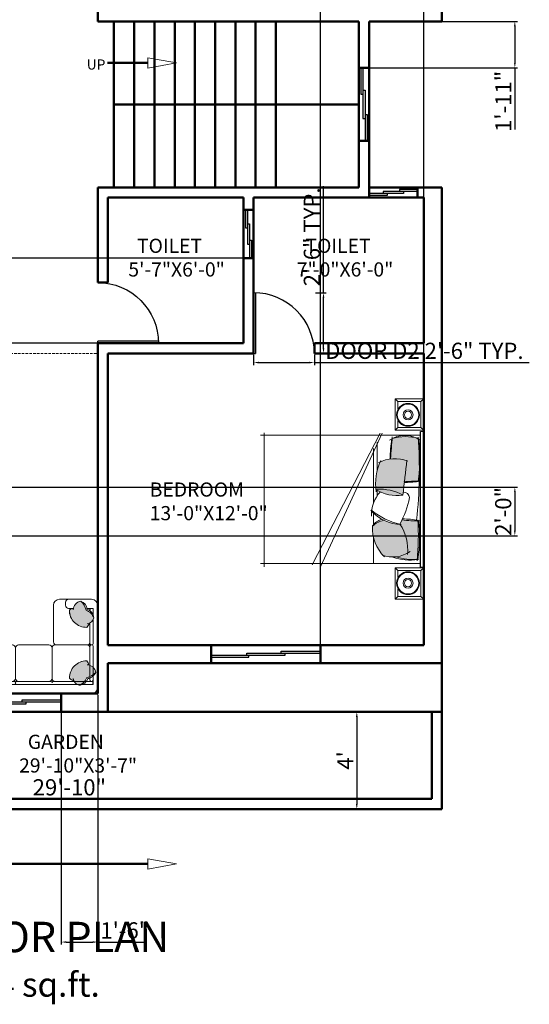
# Model space of a CAD drawing. Units: inches. Extents: x 1913 to 5309, y 1003 to 1733.
# Tile 7 of 23: x 2303 to 2555, y 1003 to 1489. Entities that reach past the tile are written whole.
import ezdxf

# ---------------------------------------------------------------- set-up
doc = ezdxf.new("R2010")
doc.units = ezdxf.units.IN
doc.linetypes.add('HIDDEN2', pattern=[0.1875, 0.125, -0.0625])
for name, color, linetype, lineweight in [('0.10', 252, 'Continuous', 9), ('0.15', 34, 'Continuous', 15), ('A-ANNO-DIMS', 2, 'Continuous', 18), ('A-ANNO-SYMB', 1, 'Continuous', 18), ('A-ANNO-TEXT', 7, 'Continuous', 18), ('A-AREA-IDEN', 3, 'Continuous', 18), ('A-DOOR', 4, 'Continuous', 25), ('A-FURN', 8, 'Continuous', 18), ('A-FURN-PATT', 8, 'Continuous', 13), ('A-GLAZ', 5, 'Continuous', 25), ('A-WALL', 7, 'Continuous', 50), ('A-WALL-OVHD', 8, 'HIDDEN2', 18)]:
    doc.layers.add(name, color=color, linetype=linetype, lineweight=lineweight)
doc.styles.get("Standard").update_dxf_attribs({"font": 'arial.ttf'})
doc.dimstyles.new('ISO-25', dxfattribs={"dimtxt": 8, "dimasz": 2.5, "dimexe": 1.25, "dimexo": 0.625, "dimtad": 1, "dimdec": 1, "dimlunit": 3, "dimtxsty": 'Standard', "dimcen": 2.5, "dimclrd": 256, "dimclrt": 1, "dimadec": 0, "dimazin": 0, "dimtfac": 1, "dimtdec": 1, "dimtmove": 0, "dimatfit": 3, "dimfxl": 1, "dimarcsym": 0})

# ---------------------------------------------------------------- blocks, each defined once
blk = doc.blocks.new("D2 2'6")
for p, q in [((0, 30), (0, 0)), ((1, 30), (1, 0)), ((0, 0), (1, 0))]:
    blk.add_line(p, q)
blk.add_arc((0, 0), 30, 0, 90)
blk = doc.blocks.new('camita')
at = {"layer": '0.10'}
for p, q in [((-0.85, -0.045), (0.85, -0.045)), ((-0.805, -0.045), (-0.805, -2.048)), ((0.805, -0.045), (0.805, -2.048)), ((-0.827, -0.521), (0.846, -1.293)), ((-0.827, -0.548), (0.824, -1.399)), ((-0.716, -0.585), (-0.355, -0.585)), ((-0.114, -0.585), (-0.049, -0.585)), ((-0.638, -0.63), (0.043, -0.63)), ((0.175, -0.63), (0.318, -0.63)), ((0.474, -0.63), (0.805, -0.63)), ((-0.835, -2), (0.846, -2))]:
    blk.add_line(p, q, dxfattribs=at)
blk.add_lwpolyline([(-0.85, -0.041), (0.85, -0.041), (0.85, 0), (-0.85, 0)], close=True, dxfattribs=at)
for centre, radius, start, end in [((-0.457, -0.236), 0.344, 147.51, 213.8336), ((-0.2, -0.227), 0.586, 163.9263, 197.1409), ((-0.364, -5.846), 5.791, 83.8073, 94.1211), ((-0.51, -1.723), 1.678, 80.1255, 98.6619), ((2.353, -0.053), 2.58, 180.1063, 184.3854), ((-1.544, -0.245), 1.333, 359.9394, 7.5533), ((1.581, -0.289), 1.335, 170.3802, 178.9914), ((-1.44, -0.061), 1.712, 352.9291, 0.3959), ((0.452, -3.067), 3, 83.9026, 93.6759), ((0.486, -1.629), 1.578, 80.1602, 98.06), ((0.029, -0.138), 0.726, 342.5841, 6.0048), ((0.133, -0.17), 0.631, 339.923, 8.7433), ((-0.054, -0.363), 0.454, 159.3026, 206.5026), ((-1.33, -9.675), 9.499, 82.2708, 84.9399), ((-0.007, -0.258), 0.0828, 100.018, 179.736), ((-0.293, -1.438), 1.29, 61.9749, 77.8435), ((0.627, -0.752), 0.551, 82.9691, 124.6739), ((0.32, -0.394), 0.404, 341.4524, 33.4512), ((0.458, -0.545), 0.584, 151.0456, 184.1497), ((-0.534, -0.339), 0.487, 327.2644, 9.0473), ((-0.199, -0.274), 0.516, 310.7395, 359.0576), ((-0.567, -0.087), 0.906, 321.6953, 346.4626), ((-1.867, -14.986), 14.632, 84.6597, 85.7516), ((-0.46, 1.486), 1.909, 260.953, 268.6517), ((0.361, -0.133), 0.51, 267.2589, 315.2997), ((-0.2, 0.064), 0.667, 244.7809, 279.0606), ((0.179, -0.272), 0.383, 224.5284, 275.2229), ((0.438, -0.483), 0.19, 193.6849, 236.7035), ((0.571, -0.432), 0.315, 192.9388, 221.9636)]:
    blk.add_arc(centre, radius, start, end, dxfattribs=at)
blk = doc.blocks.new('VELADOR')
at = {"layer": '0.15'}
for p, q in [((-0.248, 0), (-0.203, -0.045)), ((0.248, 0), (0.202, -0.045)), ((-0.203, -0.405), (-0.248, -0.45)), ((0.248, -0.45), (0.202, -0.405))]:
    blk.add_line(p, q, dxfattribs=at)
blk.add_lwpolyline([(-0.248, 0), (-0.248, -0.45), (0.248, -0.45), (0.248, 0)], close=True, dxfattribs=at)
blk.add_lwpolyline([(0.092, -0.405), (0.202, -0.405), (0.202, -0.045), (-0.203, -0.045), (-0.203, -0.405), (-0.082, -0.405)], dxfattribs=at)
for radius in [0.18, 0.169, 0.0788, 0.0563]:
    blk.add_circle((0.005, -0.247), radius, dxfattribs=at)
blk = doc.blocks.new('SOFA 1')
at = {"transparency": 33554687}
h = blk.add_hatch(color=256, dxfattribs=at)
h.dxf.hatch_style = 1
h.paths.add_polyline_path([(3723.52, 1308.63, 0.147724), (3717.76, 1305.24, 0.310469), (3722.42, 1300.4), (3722.42, 1300.25, 0.156703), (3723.62, 1297.8, 0.425821), (3734.69, 1309.08, 0.121928), (3732.05, 1310.63, 0.233216), (3728.6, 1313.59, 0.213835)])
h = blk.add_hatch(color=256, dxfattribs=at)
h.dxf.hatch_style = 1
h.paths.add_polyline_path([(3769.65, 1307.6, 0.084911), (3767.15, 1309.12, 0.046133), (3766.46, 1311.13), (3759.18, 1311.13, 0.039409), (3758.92, 1310.24, 0.165523), (3756.31, 1309.02, 0.42585), (3767.59, 1297.95, 0.121928), (3769.15, 1300.58, 0.027403), (3769.65, 1300.83)])
h.paths.add_polyline_path([(3765.34, 1313.08), (3760.4, 1313.08, 0.097704), (3759.18, 1311.13), (3766.46, 1311.13, 0.04873)])
h.paths.add_polyline_path([(3763.76, 1314.88, 0.16488), (3760.4, 1313.08), (3765.34, 1313.08, 0.051917)])
h.paths.add_polyline_path([(3771.6, 1305.17, 0.090388), (3769.65, 1307.6), (3769.65, 1300.83, 0.136035), (3771.6, 1302.77)])
h = blk.add_hatch(color=256, dxfattribs=at)
h.dxf.hatch_style = 1
h.paths.add_polyline_path([(3769.16, 1235.96, 0.122267), (3767.6, 1238.61, 0.425972), (3756.32, 1227.54, 0.165563), (3758.93, 1226.32, 0.309481), (3763.76, 1221.69, 0.002677), (3763.83, 1221.72, 0.146094), (3767.16, 1227.43, 0.212433), (3772.1, 1232.48, 0.235342)])
h = blk.add_hatch(color=256, dxfattribs=at)
h.dxf.hatch_style = 1
h.paths.add_polyline_path([(3769.16, 1225.36, 0.122267), (3767.6, 1228.01, 0.425972), (3756.32, 1216.94, 0.165563), (3758.93, 1215.72, 0.309481), (3763.76, 1211.09, 0.002677), (3763.83, 1211.12, 0.146094), (3767.16, 1216.83, 0.212433), (3772.1, 1221.88, 0.235342)])
for p, q in [((3720.45, 1316.13), (3773.58, 1316.13)), ((3777.51, 1312.19), (3777.51, 1213.72))]:
    blk.add_line(p, q, dxfattribs=at)
for points in [[(3716.51, 1312.2), (3716.51, 1291.44)], [(3722.42, 1313.08), (3722.42, 1309.23), (3722.42, 1313.08), (3726.57, 1313.08)], [(3723.21, 1311.13), (3723.93, 1311.13)], [(3729.85, 1313.08), (3745.25, 1313.08)], [(3731.82, 1311.13), (3745.25, 1311.13)], [(3746.01, 1312.3), (3746.01, 1288.55)], [(3746.01, 1310.97), (3746.01, 1311.36)], [(3768.11, 1313.08), (3746.78, 1313.08)], [(3768.87, 1311.13), (3746.78, 1311.13)], [(3771.6, 1313.08), (3767.75, 1313.08), (3771.6, 1313.08), (3771.6, 1308.93)], [(3769.66, 1287.39), (3769.65, 1312.3)], [(3771.6, 1313.08), (3771.61, 1233.74)], [(3746.01, 1288.54), (3746.01, 1308.23)], [(3769.65, 1309.43), (3769.65, 1308.71)], [(3722.42, 1300.39), (3722.42, 1297.33)], [(3720.45, 1295.38), (3718.48, 1295.38)], [(3720.45, 1287.5), (3744.09, 1287.5)], [(3747.99, 1286.6), (3767.69, 1286.6)], [(3769.66, 1263.75), (3769.66, 1285.81)], [(3746.02, 1284.63), (3746.02, 1264.94)], [(3769.66, 1277.18), (3769.66, 1263.75)], [(3746.02, 1260.99), (3746.02, 1241.3)], [(3747.99, 1262.97), (3767.69, 1262.97)], [(3769.66, 1240.12), (3769.66, 1262.18)], [(3770.43, 1262.97), (3770.82, 1262.97)], [(3746.02, 1237.36), (3746.02, 1213.74)], [(3747.99, 1239.33), (3767.69, 1239.33)], [(3769.66, 1235.71), (3769.66, 1238.54)], [(3770.43, 1239.33), (3770.82, 1239.33)], [(3769.66, 1225.11), (3769.66, 1227.82)], [(3771.61, 1223.14), (3771.61, 1230.47)], [(3755.86, 1215.72), (3758.92, 1215.72)], [(3767.76, 1215.72), (3771.61, 1215.72), (3771.61, 1219.84), (3771.61, 1215.72)], [(3769.66, 1216.5), (3769.66, 1217.22)], [(3749.97, 1209.8), (3773.58, 1209.8)], [(3753.91, 1211.77), (3753.91, 1213.74)]]:
    blk.add_lwpolyline(points, close=True, dxfattribs=at)
for points in [[(3717.76, 1305.24, -0.147724), (3723.52, 1308.63, -0.213355), (3728.59, 1313.59, 0.213355), (3723.52, 1308.63, 0.147724), (3717.76, 1305.24, -0.249545), (3722.86, 1309.34, 0.249545), (3717.75, 1305.25, 0.356779), (3723.4, 1300.28, -0.356779), (3717.76, 1305.24)], [(3734.69, 1309.08, -0.425972), (3723.62, 1297.8, -0.165552), (3722.4, 1300.4, 0.165552), (3723.62, 1297.79, 0.425972), (3734.69, 1309.07, 0.121514), (3732.07, 1310.63, -0.121514), (3734.69, 1309.08)], [(3728.58, 1313.6, -0.306333), (3732.42, 1309.31, 0.306333), (3728.58, 1313.6, 0.306674), (3722.72, 1308.89, -0.306674), (3728.58, 1313.6)], [(3763.76, 1314.88, -0.147724), (3767.15, 1309.12, -0.213355), (3772.1, 1304.05, 0.213355), (3767.15, 1309.12, 0.147724), (3763.76, 1314.88, -0.249545), (3767.86, 1309.77, 0.249545), (3763.77, 1314.89, 0.356779), (3758.8, 1309.23, -0.356779), (3763.76, 1314.88)], [(3767.6, 1297.95, -0.425972), (3756.31, 1309.01, -0.165552), (3758.92, 1310.24, 0.165552), (3756.31, 1309.02, 0.425972), (3767.59, 1297.95, 0.121514), (3769.14, 1300.57, -0.121514), (3767.6, 1297.95)], [(3772.11, 1304.06, -0.306333), (3767.83, 1300.22, 0.306333), (3772.11, 1304.06, 0.306674), (3767.4, 1309.91, -0.306674), (3772.11, 1304.06)], [(3770.44, 1286.63, -0.414214), (3769.66, 1287.4, 0.414214), (3770.44, 1286.63, 0.414214), (3769.66, 1285.83, -0.414214), (3770.44, 1286.63)], [(3748.01, 1262.99, -0.414214), (3746.05, 1264.95, 0.414214), (3748.01, 1262.97, 0.414213), (3746.05, 1261.01, -0.414213), (3748.01, 1262.99)], [(3770.44, 1262.99, -0.414214), (3769.66, 1263.77, 0.414214), (3770.44, 1262.99, 0.414214), (3769.66, 1262.19, -0.414214), (3770.44, 1262.99)], [(3770.83, 1262.97, -0.414214), (3771.61, 1262.19, 0.414214), (3770.83, 1262.99, 0.414214), (3771.61, 1263.77, -0.414214), (3770.83, 1262.97)], [(3748.01, 1239.35, -0.414214), (3746.05, 1241.31, 0.414214), (3748.01, 1239.33, 0.414213), (3746.05, 1237.37, -0.414213), (3748.01, 1239.35)], [(3767.7, 1239.33, -0.414214), (3769.66, 1237.37, 0.414214), (3767.7, 1239.35, 0.414214), (3769.66, 1241.31, -0.414214), (3767.7, 1239.33)], [(3756.32, 1227.54, -0.425972), (3767.6, 1238.61, -0.121514), (3769.16, 1235.98, 0.121514), (3767.6, 1238.61, 0.425972), (3756.32, 1227.54, 0.165552), (3758.93, 1226.32, -0.165552), (3756.32, 1227.54)], [(3772.1, 1232.5, -0.306674), (3767.41, 1226.64, 0.306674), (3772.1, 1232.5, 0.306333), (3767.84, 1236.34, -0.306333), (3772.1, 1232.5)], [(3770.44, 1239.35, -0.414214), (3769.66, 1240.13, 0.414214), (3770.44, 1239.33, 0.414214), (3769.66, 1238.55, -0.414214), (3770.44, 1239.35)], [(3770.83, 1239.33, -0.414214), (3771.61, 1238.55, 0.414214), (3770.83, 1239.35, 0.414214), (3771.61, 1240.13, -0.414214), (3770.83, 1239.33)], [(3763.78, 1221.67, 0.249545), (3767.87, 1226.78, -0.249545), (3763.76, 1221.69, -0.356779), (3758.81, 1227.32, 0.356779), (3763.77, 1221.68, 0.147724), (3767.16, 1227.43, 0.213355), (3772.11, 1232.51, -0.213355), (3767.16, 1227.43, -0.147724), (3763.78, 1221.67)], [(3756.32, 1216.94, -0.200233), (3759.49, 1224.76, 0.200233), (3756.32, 1216.94, 0.165552), (3758.93, 1215.72, -0.165552), (3756.32, 1216.94)], [(3772.1, 1221.9, -0.306674), (3767.41, 1216.04, 0.306674), (3772.1, 1221.9, -0.213355), (3767.16, 1216.83, -0.147724), (3763.77, 1211.08, 0.147724), (3767.15, 1216.83, 0.213355), (3772.1, 1221.9)], [(3763.76, 1211.09, -0.356779), (3758.81, 1216.72, 0.356779), (3763.76, 1211.09, 0.249545), (3767.87, 1216.18, -0.249545), (3763.76, 1211.09)]]:
    blk.add_lwpolyline(points, format="xyb", dxfattribs=at)
for points in [[(3722.42, 1311.91, 0.414214), (3723.2, 1311.13, -0.414214)], [(3770.43, 1313.08, 0.414214), (3769.65, 1312.3, -0.414214)], [(3771.6, 1312.3, 0.414214), (3770.82, 1313.08, -0.414214)], [(3716.51, 1297.34, 0.414214), (3718.47, 1295.38, -0.414214)], [(3716.51, 1291.45, 0.414212), (3720.44, 1287.52, -0.414212)], [(3720.44, 1295.38, 0.414214), (3722.4, 1297.34, -0.414214)], [(3746.03, 1288.56, 0.414214), (3747.99, 1286.6, 0.414213), (3746.03, 1284.64, -0.414213), (3747.99, 1286.6, -0.414214)], [(3769.66, 1284.64, 0.414214), (3767.7, 1286.6, 0.414214), (3769.66, 1288.56, -0.414214), (3767.7, 1286.6, -0.414214)], [(3769.66, 1261.01, 0.414214), (3767.7, 1262.97, 0.414214), (3769.66, 1264.93, -0.414214), (3767.7, 1262.97, -0.414214)], [(3772.13, 1221.9, 0.306333), (3767.84, 1225.74, -0.306333)], [(3769.16, 1225.36, 0.071861), (3768.39, 1227.01, -0.071861)], [(3755.87, 1215.72, 0.414214), (3753.91, 1213.76, -0.414214)], [(3769.66, 1216.52, 0.414214), (3770.44, 1215.74, -0.414214)], [(3770.83, 1215.74, 0.414214), (3771.61, 1216.52, -0.414214)], [(3746.05, 1213.76, 0.414212), (3749.98, 1209.82, -0.414212)], [(3755.87, 1209.8, -0.414214), (3753.91, 1211.76, 0.414214)]]:
    blk.add_lwpolyline(points, format="xyb", close=True, dxfattribs=at)
for centre, radius, start, end in [((3720.44, 1312.2), 3.93, 90.00019, 179.99981), ((3720.44, 1312.19), 3.94, 89.91581, 179.91542), ((3744.09, 1309.21), 1.92, 358.76597, 90.51112), ((3745.22, 1312.29), 0.789, 0.84252, 90.84253), ((3745.24, 1311.91), 0.777, 270, 0), ((3745.24, 1311.91), 0.777, 270, 0), ((3746.8, 1312.29), 0.789, 89.15747, 179.15748), ((3746.79, 1311.91), 0.777, 180, 270), ((3746.79, 1311.91), 0.777, 180, 270), ((3747.93, 1309.21), 1.92, 89.48888, 181.23403), ((3768.87, 1312.3), 0.777, 360, 90), ((3768.87, 1311.91), 0.777, 270, 0), ((3773.58, 1312.2), 3.93, 0.00019, 89.99981), ((3773.57, 1312.19), 3.94, 359.91581, 89.91542), ((3744.08, 1289.48), 1.96, 270, 360), ((3744.08, 1289.48), 1.96, 270, 360), ((3773.58, 1213.73), 3.93, 270.00019, 359.99981), ((3773.59, 1213.73), 3.93, 269.91556, 359.91517)]:
    blk.add_arc(centre, radius, start, end, dxfattribs=at)
blk = doc.blocks.new('*D25')
at = {"layer": 'A-ANNO-DIMS', "color": 0, "lineweight": -2, "transparency": 16777216}
for p, q in [((2469.32, 1144.46), (2469.32, 1101.46)), ((2469.94, 1146.96), (2470.57, 1146.96)), ((2469.94, 1098.96), (2470.57, 1098.96))]:
    blk.add_line(p, q, dxfattribs=at)
at = {"layer": 'A-ANNO-DIMS', "color": 0, "transparency": 16777216}
for points in [[(2468.9, 1144.46), (2469.73, 1144.46), (2469.32, 1146.96)], [(2468.9, 1101.46), (2469.73, 1101.46), (2469.32, 1098.96)]]:
    blk.add_solid(points, dxfattribs=at)
at = {"layer": 'Defpoints', "color": 0, "transparency": 16777216}
for p in [(2469.32, 1146.96), (2469.32, 1098.96), (2469.32, 1098.96)]:
    blk.add_point(p, dxfattribs=at)
at = {"layer": 'A-ANNO-DIMS', "color": 0, "transparency": 16777216, "insert": (2464.69, 1122.96), "char_height": 8, "attachment_point": 5, "rotation": 90}
blk.add_mtext("4'", dxfattribs=at)
blk = doc.blocks.new('*D21')
at = {"layer": 'A-ANNO-DIMS', "color": 0, "lineweight": -2, "transparency": 16777216}
for p, q in [((2148.37, 1104.59), (2148.37, 1105.21)), ((2503.87, 1103.96), (2150.87, 1103.96)), ((2506.37, 1104.59), (2506.37, 1105.21))]:
    blk.add_line(p, q, dxfattribs=at)
at = {"layer": 'A-ANNO-DIMS', "color": 0, "transparency": 16777216}
for points in [[(2150.87, 1104.38), (2150.87, 1103.55), (2148.37, 1103.96)], [(2503.87, 1104.38), (2503.87, 1103.55), (2506.37, 1103.96)]]:
    blk.add_solid(points, dxfattribs=at)
at = {"layer": 'Defpoints', "color": 0, "transparency": 16777216}
for p in [(2148.37, 1103.96), (2148.37, 1103.96), (2506.37, 1103.96)]:
    blk.add_point(p, dxfattribs=at)
at = {"layer": 'A-ANNO-DIMS', "color": 0, "transparency": 16777216, "insert": (2327.37, 1108.67), "char_height": 8, "attachment_point": 5}
blk.add_mtext('29\'-10"', dxfattribs=at)
blk = doc.blocks.new('WIN-24')
for p, q in [((0, 15), (0, 24)), ((1, 7), (1, 24)), ((1, 15), (0, 15)), ((2, 17), (1, 17)), ((2, 0), (2, 17)), ((2, 7), (1, 7)), ((3, 9), (2, 9)), ((3, 0), (3, 9))]:
    blk.add_line(p, q)
blk = doc.blocks.new('WIN-54')
for p, q in [((0, 54), (0, 35)), ((1, 54), (1, 17)), ((0, 35), (1, 35)), ((1, 36), (2, 36)), ((2, 36), (2, 0)), ((1, 17), (2, 17)), ((2, 19), (3, 19)), ((3, 19), (3, 0))]:
    blk.add_line(p, q)
blk = doc.blocks.new('WIN-36')
for p, q in [((0, 23), (0, 36)), ((1, 11), (1, 36)), ((2, 25), (1, 25)), ((2, 0), (2, 25)), ((1, 23), (0, 23)), ((2, 11), (1, 11)), ((3, 13), (2, 13)), ((3, 0), (3, 13))]:
    blk.add_line(p, q)
blk = doc.blocks.new('*D73')
at = {"layer": 'A-ANNO-DIMS', "color": 0, "lineweight": -2, "transparency": 16777216}
for p, q in [((2418.37, 1323.34), (2418.37, 1318.21)), ((2448.37, 1323.34), (2448.37, 1318.21))]:
    blk.add_line(p, q, dxfattribs=at)
at = {"layer": 'A-ANNO-DIMS', "lineweight": -2, "transparency": 16777216}
for p, q in [((2420.87, 1319.46), (2445.87, 1319.46)), ((2448.37, 1319.46), (2554.51, 1319.46))]:
    blk.add_line(p, q, dxfattribs=at)
at = {"layer": 'A-ANNO-DIMS', "transparency": 16777216}
for points in [[(2420.87, 1319.88), (2420.87, 1319.05), (2418.37, 1319.46)], [(2445.87, 1319.88), (2445.87, 1319.05), (2448.37, 1319.46)]]:
    blk.add_solid(points, dxfattribs=at)
at = {"layer": 'Defpoints', "color": 0, "transparency": 16777216}
for p in [(2418.37, 1323.96), (2448.37, 1323.96), (2448.37, 1319.46)]:
    blk.add_point(p, dxfattribs=at)
at = {"layer": 'A-ANNO-DIMS', "color": 1, "transparency": 16777216, "insert": (2502.69, 1324.23), "char_height": 8, "attachment_point": 5}
blk.add_mtext('DOOR D2 2\'-6" TYP.', dxfattribs=at)
blk = doc.blocks.new('*D74')
at = {"layer": 'A-ANNO-DIMS', "lineweight": -2, "transparency": 16777216}
for p, q in [((2452.87, 1353.96), (2452.87, 1406.61)), ((2452.87, 1326.46), (2452.87, 1351.46))]:
    blk.add_line(p, q, dxfattribs=at)
at = {"layer": 'A-ANNO-DIMS', "color": 0, "lineweight": -2, "transparency": 16777216}
for p, q in [((2449, 1353.96), (2454.12, 1353.96)), ((2449, 1323.96), (2454.12, 1323.96))]:
    blk.add_line(p, q, dxfattribs=at)
at = {"layer": 'A-ANNO-DIMS', "transparency": 16777216}
for points in [[(2452.46, 1351.46), (2453.29, 1351.46), (2452.87, 1353.96)], [(2452.46, 1326.46), (2453.29, 1326.46), (2452.87, 1323.96)]]:
    blk.add_solid(points, dxfattribs=at)
at = {"layer": 'Defpoints', "color": 0, "transparency": 16777216}
for p in [(2448.37, 1353.96), (2452.87, 1353.96), (2448.37, 1323.96)]:
    blk.add_point(p, dxfattribs=at)
at = {"layer": 'A-ANNO-DIMS', "color": 1, "transparency": 16777216, "insert": (2448.16, 1381.54), "char_height": 8, "attachment_point": 5, "rotation": 90}
blk.add_mtext('2\'-6" TYP.', dxfattribs=at)
blk = doc.blocks.new('*D96')
at = {"layer": 'A-ANNO-DIMS', "color": 0, "lineweight": -2, "transparency": 16777216}
for p, q in [((2476, 1487.96), (2548.62, 1487.96)), ((2476, 1464.96), (2548.62, 1464.96))]:
    blk.add_line(p, q, dxfattribs=at)
at = {"layer": 'A-ANNO-DIMS', "lineweight": -2, "transparency": 16777216}
for p, q in [((2547.37, 1485.46), (2547.37, 1467.46)), ((2547.37, 1464.96), (2547.37, 1434.49))]:
    blk.add_line(p, q, dxfattribs=at)
at = {"layer": 'A-ANNO-DIMS', "transparency": 16777216}
for points in [[(2546.96, 1485.46), (2547.79, 1485.46), (2547.37, 1487.96)], [(2546.96, 1467.46), (2547.79, 1467.46), (2547.37, 1464.96)]]:
    blk.add_solid(points, dxfattribs=at)
at = {"layer": 'Defpoints', "color": 0, "transparency": 16777216}
for p in [(2475.37, 1487.96), (2475.37, 1464.96), (2547.37, 1464.96)]:
    blk.add_point(p, dxfattribs=at)
at = {"layer": 'A-ANNO-DIMS', "color": 1, "transparency": 16777216, "insert": (2542.73, 1448.47), "char_height": 8, "attachment_point": 5, "rotation": 90}
blk.add_mtext('1\'-11"', dxfattribs=at)
blk = doc.blocks.new('*D97')
at = {"layer": 'A-ANNO-DIMS', "color": 0, "lineweight": -2, "transparency": 16777216}
for p, q in [((2323.37, 1155.34), (2323.37, 1032.04)), ((2341.37, 1155.34), (2341.37, 1032.04))]:
    blk.add_line(p, q, dxfattribs=at)
at = {"layer": 'A-ANNO-DIMS', "lineweight": -2, "transparency": 16777216}
for p, q in [((2325.87, 1033.29), (2338.87, 1033.29)), ((2341.37, 1033.29), (2365.64, 1033.29))]:
    blk.add_line(p, q, dxfattribs=at)
at = {"layer": 'A-ANNO-DIMS', "transparency": 16777216}
for points in [[(2325.87, 1033.7), (2325.87, 1032.87), (2323.37, 1033.29)], [(2338.87, 1033.7), (2338.87, 1032.87), (2341.37, 1033.29)]]:
    blk.add_solid(points, dxfattribs=at)
at = {"layer": 'Defpoints', "color": 0, "transparency": 16777216}
for p in [(2323.37, 1155.96), (2341.37, 1155.96), (2341.37, 1033.29)]:
    blk.add_point(p, dxfattribs=at)
at = {"layer": 'A-ANNO-DIMS', "color": 1, "transparency": 16777216, "insert": (2354.75, 1038), "char_height": 8, "attachment_point": 5}
blk.add_mtext('1\'-6"', dxfattribs=at)
blk = doc.blocks.new('*D99')
at = {"layer": 'A-ANNO-DIMS', "color": 0, "lineweight": -2, "transparency": 16777216}
for p, q in [((2451.37, 1180.59), (2451.37, 1724.21)), ((2502.37, 1180.59), (2502.37, 1724.21))]:
    blk.add_line(p, q, dxfattribs=at)
at = {"layer": 'A-ANNO-DIMS', "lineweight": -2, "transparency": 16777216}
blk.add_line((2453.87, 1722.96), (2499.87, 1722.96), dxfattribs=at)
at = {"layer": 'A-ANNO-DIMS', "transparency": 16777216}
for points in [[(2453.87, 1723.38), (2453.87, 1722.55), (2451.37, 1722.96)], [(2499.87, 1723.38), (2499.87, 1722.55), (2502.37, 1722.96)]]:
    blk.add_solid(points, dxfattribs=at)
at = {"layer": 'Defpoints', "color": 0, "transparency": 16777216}
for p in [(2502.37, 1722.96), (2451.37, 1179.96), (2502.37, 1179.96)]:
    blk.add_point(p, dxfattribs=at)
at = {"layer": 'A-ANNO-DIMS', "color": 1, "transparency": 16777216, "insert": (2476.87, 1727.68), "char_height": 8, "attachment_point": 5}
blk.add_mtext('4\'-3"', dxfattribs=at)
blk = doc.blocks.new('*D101')
at = {"layer": 'A-ANNO-DIMS', "color": 0, "lineweight": -2, "transparency": 16777216}
for p, q in [((2158, 1257.96), (2548.62, 1257.96)), ((2158, 1233.96), (2548.62, 1233.96))]:
    blk.add_line(p, q, dxfattribs=at)
at = {"layer": 'A-ANNO-DIMS', "lineweight": -2, "transparency": 16777216}
blk.add_line((2547.37, 1255.46), (2547.37, 1236.46), dxfattribs=at)
at = {"layer": 'A-ANNO-DIMS', "transparency": 16777216}
for points in [[(2546.96, 1255.46), (2547.79, 1255.46), (2547.37, 1257.96)], [(2546.96, 1236.46), (2547.79, 1236.46), (2547.37, 1233.96)]]:
    blk.add_solid(points, dxfattribs=at)
at = {"layer": 'Defpoints', "color": 0, "transparency": 16777216}
for p in [(2157.37, 1257.96), (2157.37, 1233.96), (2547.37, 1233.96)]:
    blk.add_point(p, dxfattribs=at)
at = {"layer": 'A-ANNO-DIMS', "color": 1, "transparency": 16777216, "insert": (2542.66, 1245.96), "char_height": 8, "attachment_point": 5, "rotation": 90}
blk.add_mtext('2\'-0"', dxfattribs=at)
blk = doc.blocks.new('*D102')
at = {"layer": 'A-ANNO-DIMS', "color": 0, "lineweight": -2, "transparency": 16777216}
for p, q in [((2412.75, 1370.96), (1922.12, 1370.96)), ((2412.75, 1328.96), (1922.12, 1328.96))]:
    blk.add_line(p, q, dxfattribs=at)
at = {"layer": 'A-ANNO-DIMS', "lineweight": -2, "transparency": 16777216}
blk.add_line((1923.37, 1331.46), (1923.37, 1368.46), dxfattribs=at)
at = {"layer": 'A-ANNO-DIMS', "transparency": 16777216}
for points in [[(1922.96, 1368.46), (1923.79, 1368.46), (1923.37, 1370.96)], [(1922.96, 1331.46), (1923.79, 1331.46), (1923.37, 1328.96)]]:
    blk.add_solid(points, dxfattribs=at)
at = {"layer": 'Defpoints', "color": 0, "transparency": 16777216}
for p in [(1923.37, 1370.96), (2413.37, 1370.96), (2413.37, 1328.96)]:
    blk.add_point(p, dxfattribs=at)
at = {"layer": 'A-ANNO-DIMS', "color": 1, "transparency": 16777216, "insert": (1918.66, 1349.96), "char_height": 8, "attachment_point": 5, "rotation": 90}
blk.add_mtext('3\'-6"', dxfattribs=at)

msp = doc.modelspace()

# ---------------------------------------------------------------- hatches: boundary and pattern name
at = {"layer": 'A-FURN-PATT'}
h = msp.add_hatch(color=256, dxfattribs=at)
h.dxf.hatch_style = 1
h.paths.add_polyline_path([(2485.94, 1271.86, -0.113891), (2493.94, 1270.99, -0.006967), (2492.87, 1260.63, -0.016701), (2499.65, 1260.9, 0.015442), (2500.21, 1264.94, 0.01851), (2499.69, 1281.81, 0.020657), (2498.69, 1282.31, 0.131047), (2486.8, 1281.93, -0.004387)])
h.paths.add_polyline_path([(2491.68, 1241.76, -0.011742), (2490.61, 1239.63, -0.175864), (2494.37, 1225.32, -0.098488), (2488.43, 1223.51, 0.094792), (2499.1, 1222.29, 0.040212), (2499.49, 1241.25, -0.029051)])
h = msp.add_hatch(color=256, dxfattribs=at)
h.dxf.hatch_style = 1
h.paths.add_polyline_path([(2478.8, 1256.74, 0.181694), (2492.03, 1254.04, 0.011408), (2493.94, 1270.99, 0.189536), (2480.86, 1270.47, 0.134508)])
h.paths.add_polyline_path([(2490.7, 1239.49, -0.104045), (2482.6, 1241.56, 0.127326), (2477.09, 1238.7, 0.202559), (2482.48, 1224.04, 0.194952), (2494.37, 1225.32, 0.173835)])

# ---------------------------------------------------------------- linework, layer by layer
at = {"layer": 'A-ANNO-SYMB'}
for points in [[(2380.2, 1467.46), (2366.04, 1470.02), (2366.04, 1464.91)], [(2380.2, 1071.84), (2366.04, 1074.39), (2366.04, 1069.29)]]:
    msp.add_lwpolyline(points, close=True, dxfattribs=at)
at = {"layer": 'A-WALL'}
for p, q in [((2511.37, 1686.96), (2511.37, 1487.96)), ((2341.37, 1492.96), (2341.37, 1487.96)), ((2341.37, 1487.96), (2470.37, 1487.96)), ((2349.37, 1487.96), (2349.37, 1405.96)), ((2359.37, 1487.96), (2359.37, 1405.96)), ((2369.37, 1487.96), (2369.37, 1405.96)), ((2379.37, 1487.96), (2379.37, 1405.96)), ((2389.37, 1487.96), (2389.37, 1405.96)), ((2399.37, 1487.96), (2399.37, 1405.96)), ((2409.37, 1487.96), (2409.37, 1405.96)), ((2419.37, 1487.96), (2419.37, 1405.96)), ((2429.37, 1487.96), (2429.37, 1405.96)), ((2470.37, 1487.96), (2470.37, 1405.96)), ((2475.37, 1487.96), (2511.37, 1487.96)), ((2475.37, 1487.96), (2475.37, 1400.96)), ((2366.04, 1467.46), (2346.12, 1467.46)), ((2475.37, 1464.96), (2470.37, 1464.96)), ((2470.37, 1446.96), (2349.37, 1446.96)), ((2475.37, 1428.96), (2470.37, 1428.96)), ((2341.37, 1405.96), (2470.37, 1405.96)), ((2341.37, 1405.96), (2341.37, 1358.96)), ((2475.37, 1405.96), (2511.37, 1405.96)), ((2499.37, 1405.96), (2499.37, 1400.96)), ((2511.37, 1405.96), (2511.37, 1098.96)), ((2346.37, 1400.96), (2413.37, 1400.96)), ((2346.37, 1400.96), (2346.37, 1358.96)), ((2413.37, 1400.96), (2413.37, 1328.96)), ((2418.37, 1400.96), (2502.37, 1400.96)), ((2418.37, 1400.96), (2418.37, 1323.96)), ((2502.37, 1400.96), (2502.37, 1328.96)), ((2413.37, 1394.96), (2418.37, 1394.96)), ((2413.37, 1370.96), (2418.37, 1370.96)), ((2341.37, 1358.96), (2346.37, 1358.96)), ((2341.37, 1328.96), (2413.37, 1328.96)), ((2341.37, 1328.96), (2341.37, 1155.96)), ((2448.37, 1328.96), (2502.37, 1328.96)), ((2448.37, 1328.96), (2448.37, 1323.96)), ((2346.37, 1323.96), (2418.37, 1323.96)), ((2346.37, 1323.96), (2346.37, 1179.96)), ((2448.37, 1323.96), (2502.37, 1323.96)), ((2502.37, 1323.96), (2502.37, 1179.96)), ((2346.37, 1179.96), (2502.37, 1179.96)), ((2397.37, 1179.96), (2397.37, 1170.96)), ((2451.37, 1179.96), (2451.37, 1170.96)), ((2346.37, 1170.96), (2511.37, 1170.96)), ((2346.37, 1170.96), (2346.37, 1146.96)), ((2157.37, 1155.96), (2341.37, 1155.96)), ((2323.37, 1155.96), (2323.37, 1146.96)), ((2148.37, 1146.96), (2511.37, 1146.96)), ((2506.37, 1146.96), (2506.37, 1103.96)), ((2124.37, 1103.96), (2506.37, 1103.96)), ((2511.37, 1098.96), (2124.37, 1098.96)), ((2366.04, 1071.84), (2266.22, 1071.84))]:
    msp.add_line(p, q, dxfattribs=at)
at = {"layer": 'A-WALL-OVHD', "ltscale": 10}
for p, q in [((2281.37, 1328.96), (2341.37, 1328.96)), ((2281.37, 1323.96), (2341.37, 1323.96))]:
    msp.add_line(p, q, dxfattribs=at)

# ---------------------------------------------------------------- block references
at = {"layer": 'A-DOOR', "xscale": -1, "rotation": 270}
msp.add_blockref("D2 2'6", (2341.37, 1328.96), dxfattribs=at)
at = {"layer": 'A-DOOR'}
msp.add_blockref("D2 2'6", (2418.37, 1323.96), dxfattribs=at)
at = {"layer": 'A-FURN'}
for name, p, xscale, yscale, zscale, rotation in [('VELADOR', (2502.37, 1293.8), 31.41542173157097, 31.41542173157097, 31.41542173157097, 270), ('camita', (2502.37, 1251.96), 39.375, 39.375, 39.375, 270), ('VELADOR', (2502.37, 1210.35), -31.41542173157097, 31.41542173157097, 31.41542173157097, 269.9999999999999), ('SOFA 1', (1335.32, 4043.51), 0.7644053585719659, 0.7644053585719659, 0.7644053585719659, 270)]:
    msp.add_blockref(name, p, dxfattribs=dict(at, xscale=xscale, yscale=yscale, zscale=zscale, rotation=rotation))
at = {"layer": 'A-GLAZ'}
for name, p, rotation in [('WIN-36', (2474.37, 1464.96), 180), ('WIN-24', (2499.37, 1401.96), 89.99999999999156), ('WIN-24', (2417.37, 1394.96), 180), ('WIN-54', (2451, 1173.98), 90.04407578688497), ('WIN-54', (2323, 1149.98), 90.04407578688537)]:
    msp.add_blockref(name, p, dxfattribs=dict(at, rotation=rotation))

# ---------------------------------------------------------------- texts
at = {"layer": 'A-ANNO-TEXT', "attachment_point": 1}
for s, width, insert, char_height in [('UP', 10.7355, (2335.93, 1469.16), 5), ('GROUND FLOOR PLAN\\P{\\H0.8x;SLAB AREA = 1914 sq.ft.}', 253.2094, (2164.58, 1043.3), 15)]:
    msp.add_mtext_dynamic_manual_height_columns(s, width=width, gutter_width=12.5, heights=[0], dxfattribs=dict(at, insert=insert, char_height=char_height))
at = {"layer": 'A-AREA-IDEN', "char_height": 7, "attachment_point": 1}
for s, insert in [('  TOILET\\P5\'-7"X6\'-0"', (2356.49, 1380.62)), ('  TOILET\\P7\'-0"X6\'-0"', (2439.69, 1380.62)), ('BEDROOM\\P13\'-0"X12\'-0"', (2367.05, 1260.26)), ('  GARDEN\\P29\'-10"X3\'-7"', (2302.55, 1135.66))]:
    msp.add_mtext_dynamic_manual_height_columns(s, width=86.9528, gutter_width=12.5, heights=[0], dxfattribs=dict(at, insert=insert))

# ---------------------------------------------------------------- dimensions: what is measured, and where the dimension line sits
at = {"layer": 'A-ANNO-DIMS'}
for base, p1, p2, override, picture, middle in [((2502.37, 1722.96), (2451.37, 1179.96), (2502.37, 1179.96), {"dimdec": 1, "dimlfac": 1, "dimrnd": 0, "dimzin": 1, "dimdsep": 46, "dimlunit": 4, "dimfrac": 2}, '*D99', (2476.87, 1727.68)), ((2341.37, 1033.29), (2323.37, 1155.96), (2341.37, 1155.96), {"dimdec": 1, "dimlfac": 1, "dimrnd": 0, "dimzin": 1, "dimdsep": 46, "dimlunit": 4, "dimfrac": 2}, '*D97', (2354.75, 1038)), ((2148.37, 1103.96), (2506.37, 1103.96), (2148.37, 1103.96), {"dimclrd": 0, "dimclre": 0, "dimclrt": 0}, '*D21', (2327.37, 1108.67))]:
    dim = msp.add_linear_dim(base=base, p1=p1, p2=p2, dimstyle='ISO-25', override=override, dxfattribs=at)
    dim.commit()
    dim.dimension.update_dxf_attribs({"geometry": picture, "text_midpoint": middle})
for base, p1, p2, override, picture, middle in [((2547.37, 1464.96), (2475.37, 1487.96), (2475.37, 1464.96), {"dimdec": 1, "dimlfac": 1, "dimrnd": 0, "dimzin": 1, "dimdsep": 46, "dimlunit": 4, "dimfrac": 2}, '*D96', (2542.73, 1448.47)), ((1923.37, 1370.96), (2413.37, 1328.96), (2413.37, 1370.96), {"dimdec": 1, "dimlfac": 1, "dimrnd": 0, "dimzin": 1, "dimdsep": 46, "dimlunit": 4, "dimfrac": 2}, '*D102', (1918.66, 1349.96)), ((2547.37, 1233.96), (2157.37, 1257.96), (2157.37, 1233.96), {"dimdec": 1, "dimlfac": 1, "dimrnd": 0, "dimzin": 1, "dimdsep": 46, "dimlunit": 4, "dimfrac": 2}, '*D101', (2542.66, 1245.96)), ((2469.32, 1098.96), (2469.32, 1146.96), (2469.32, 1098.96), {"dimclrd": 0, "dimclre": 0, "dimclrt": 0}, '*D25', (2464.69, 1122.96))]:
    dim = msp.add_linear_dim(base=base, p1=p1, p2=p2, angle=90, dimstyle='ISO-25', override=override, dxfattribs=at)
    dim.commit()
    dim.dimension.update_dxf_attribs({"geometry": picture, "text_midpoint": middle})
dim = msp.add_linear_dim(base=(2452.87, 1353.96), p1=(2448.37, 1323.96), p2=(2448.37, 1353.96), angle=90, text='<> TYP.', dimstyle='ISO-25', override={"dimdec": 1, "dimrnd": 0, "dimzin": 1, "dimlunit": 4, "dimfrac": 2}, dxfattribs=at)
dim.commit()
dim.dimension.update_dxf_attribs({"geometry": '*D74', "text_midpoint": (2448.16, 1381.54)})
dim = msp.add_linear_dim(base=(2448.37, 1319.46), p1=(2418.37, 1323.96), p2=(2448.37, 1323.96), text='DOOR D2 <> TYP.', dimstyle='ISO-25', override={"dimdec": 1, "dimrnd": 0, "dimzin": 1, "dimlunit": 4, "dimfrac": 2}, dxfattribs=at)
dim.commit()
dim.dimension.update_dxf_attribs({"geometry": '*D73', "text_midpoint": (2502.69, 1324.23)})

doc.saveas('drawing.dxf')
